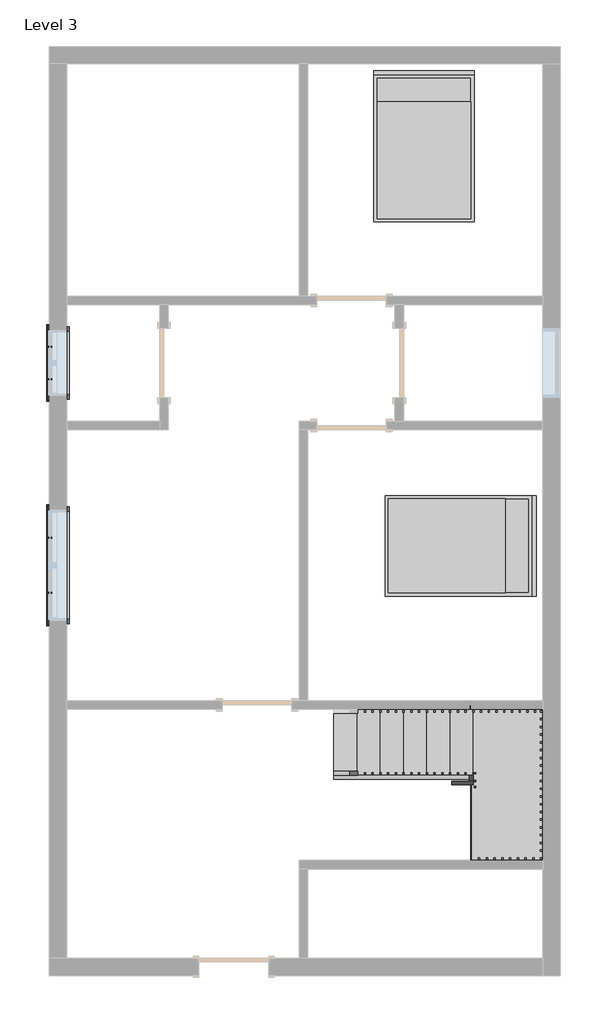
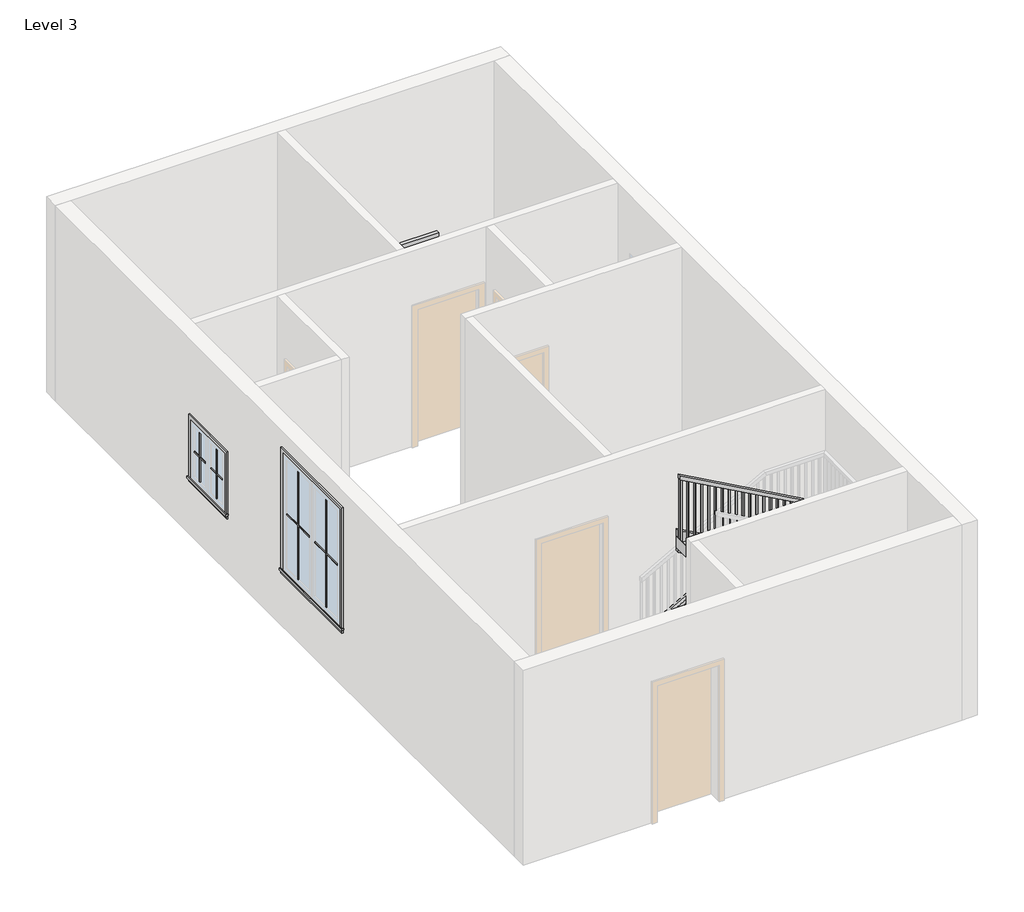
# One storey, part 2 of 2: 8 proxies, 6 members, 2 furniture elements, 1 railing, 1 stair flight.
"""IFC4 building model written with IfcOpenShell, lengths in millimetres."""

from ifc_helpers import new_model, si_unit, frame, origin, place, context, project, spatial, polyline, outline, extrude, faceted_brep, transform, mapped, element, save
from components import muntin_pattern_2x2_muntin_pattern_2x2_b3fe6957, muntin_pattern_2x2_muntin_pattern_2x2_3e0ecaf2, muntin_pattern_2x2_muntin_pattern_2x2_bff912c5, muntin_pattern_2x2_muntin_pattern_2x2_c2194282, trim_window_exterior_flat_with_sill_41619996, trim_window_exterior_flat_with_sill_e04b3088, trim_window_interior_flat_picture_frame_51c85655, trim_window_interior_flat_picture_frame_2a7685fe, bed_17739_bed_17739_15c61121, stair_flight_fe7d2e61

model = new_model("IFC4")

# Units and contexts
model_context = context("Model", 3, world=origin())
ifc_project = project(units=[si_unit("LENGTHUNIT", "METRE", prefix="MILLI")], contexts=[model_context])

# Site, building, storey
site = spatial("IfcSite", under=ifc_project)
building = spatial("IfcBuilding", under=site)
storey = spatial("IfcBuildingStorey", under=building, Name="Level 3", Elevation=3200.4)

# Proxies
placement = place(None, origin())
muntin_pattern_2x2_muntin_pattern_2x2_shape = muntin_pattern_2x2_muntin_pattern_2x2_b3fe6957(model_context)
element("IfcBuildingElementProxy", 1, Name="Muntin Pattern_2x2 : Muntin Pattern_2x2", ObjectType="Muntin Pattern_2x2 : Muntin Pattern_2x2", at=placement, inside=storey, context=model_context, shape_type="MappedRepresentation", body=[
    mapped(muntin_pattern_2x2_muntin_pattern_2x2_shape, transform((-4603.815747, 2266.9810985, 4184.65), x_axis=(0.0, 1.0, 0.0), y_axis=(-1.0, 0.0, 0.0), z_axis=(0.0, 0.0, 1.0))),
])
muntin_pattern_2x2_muntin_pattern_2x2_2_shape = muntin_pattern_2x2_muntin_pattern_2x2_3e0ecaf2(model_context)
element("IfcBuildingElementProxy", 2, Name="Muntin Pattern_2x2 : Muntin Pattern_2x2", ObjectType="Muntin Pattern_2x2 : Muntin Pattern_2x2", at=placement, inside=storey, context=model_context, shape_type="MappedRepresentation", body=[
    mapped(muntin_pattern_2x2_muntin_pattern_2x2_2_shape, transform((-4603.815747, 2695.6060985, 4184.65), x_axis=(0.0, -1.0, 0.0), y_axis=(1.0, 0.0, 0.0), z_axis=(0.0, 0.0, 1.0))),
])
muntin_pattern_2x2_muntin_pattern_2x2_3_shape = muntin_pattern_2x2_muntin_pattern_2x2_bff912c5(model_context)
element("IfcBuildingElementProxy", 3, Name="Muntin Pattern_2x2 : Muntin Pattern_2x2", ObjectType="Muntin Pattern_2x2 : Muntin Pattern_2x2", at=placement, inside=storey, context=model_context, shape_type="MappedRepresentation", body=[
    mapped(muntin_pattern_2x2_muntin_pattern_2x2_3_shape, transform((-4603.815747, -533.3689015, 4184.65), x_axis=(0.0, 1.0, 0.0), y_axis=(-1.0, 0.0, 0.0), z_axis=(0.0, 0.0, 1.0))),
])
muntin_pattern_2x2_muntin_pattern_2x2_4_shape = muntin_pattern_2x2_muntin_pattern_2x2_c2194282(model_context)
element("IfcBuildingElementProxy", 4, Name="Muntin Pattern_2x2 : Muntin Pattern_2x2", ObjectType="Muntin Pattern_2x2 : Muntin Pattern_2x2", at=placement, inside=storey, context=model_context, shape_type="MappedRepresentation", body=[
    mapped(muntin_pattern_2x2_muntin_pattern_2x2_4_shape, transform((-4603.815747, 187.3560985, 4184.65), x_axis=(0.0, -1.0, 0.0), y_axis=(1.0, 0.0, 0.0), z_axis=(0.0, 0.0, 1.0))),
])
trim_window_exterior_flat_with_sill_shape = trim_window_exterior_flat_with_sill_41619996(model_context)
element("IfcBuildingElementProxy", 5, Name="Trim-Window-Exterior-Flat : with Sill", ObjectType="Trim-Window-Exterior-Flat : with Sill", at=placement, inside=storey, context=model_context, shape_type="MappedRepresentation", body=[
    mapped(trim_window_exterior_flat_with_sill_shape, transform((-4613.340747, 2481.2935985, 5029.2), x_axis=(0.0, -1.0, 0.0), y_axis=(0.0, 0.0, 1.0), z_axis=(-1.0, 0.0, 0.0))),
])
trim_window_exterior_flat_with_sill_2_shape = trim_window_exterior_flat_with_sill_e04b3088(model_context)
element("IfcBuildingElementProxy", 6, Name="Trim-Window-Exterior-Flat : with Sill", ObjectType="Trim-Window-Exterior-Flat : with Sill", at=placement, inside=storey, context=model_context, shape_type="MappedRepresentation", body=[
    mapped(trim_window_exterior_flat_with_sill_2_shape, transform((-4613.340747, -173.0064015, 5943.6), x_axis=(0.0, -1.0, 0.0), y_axis=(0.0, 0.0, 1.0), z_axis=(-1.0, 0.0, 0.0))),
])
trim_window_interior_flat_picture_frame_shape = trim_window_interior_flat_picture_frame_51c85655(model_context)
element("IfcBuildingElementProxy", 7, Name="Trim-Window-Interior-Flat : Picture Frame", ObjectType="Trim-Window-Interior-Flat : Picture Frame", at=placement, inside=storey, context=model_context, shape_type="MappedRepresentation", body=[
    mapped(trim_window_interior_flat_picture_frame_shape, transform((-4384.740747, 2481.2935985, 5029.2), x_axis=(0.0, 1.0, 0.0), y_axis=(0.0, 0.0, 1.0), z_axis=(1.0, 0.0, 0.0))),
])
trim_window_interior_flat_picture_frame_2_shape = trim_window_interior_flat_picture_frame_2a7685fe(model_context)
element("IfcBuildingElementProxy", 8, Name="Trim-Window-Interior-Flat : Picture Frame", ObjectType="Trim-Window-Interior-Flat : Picture Frame", at=placement, inside=storey, context=model_context, shape_type="MappedRepresentation", body=[
    mapped(trim_window_interior_flat_picture_frame_2_shape, transform((-4384.740747, -173.0064015, 5943.6), x_axis=(0.0, 1.0, 0.0), y_axis=(0.0, 0.0, 1.0), z_axis=(1.0, 0.0, 0.0))),
])

# Furniture
bed_17739_bed_17739_shape = bed_17739_bed_17739_15c61121(model_context)
element("IfcFurniture", 9, ObjectType="Bed_17739 : Bed_17739", at=placement, inside=storey, context=model_context, shape_type="MappedRepresentation", body=[
    mapped(bed_17739_bed_17739_shape, transform((301.559253, 5300.6935985, 3200.4), x_axis=(1.0, 0.0, 0.0), y_axis=(0.0, 1.0, 0.0), z_axis=(0.0, 0.0, 1.0))),
])
element("IfcFurniture", 10, ObjectType="Bed_17739 : Bed_17739", at=placement, inside=storey, context=model_context, shape_type="MappedRepresentation", body=[
    mapped(bed_17739_bed_17739_shape, transform((758.759253, 80.9935985, 3200.4), x_axis=(0.0, -1.0, 0.0), y_axis=(1.0, 0.0, 0.0), z_axis=(0.0, 0.0, 1.0))),
])

# Members
element("IfcMember", 11, ObjectType="Stringer - 2\" Width", at=placement, inside=storey, context=model_context, shape_type="SweptSolid", body=[
    extrude(outline(polyline([(3407.9983948, -879.540747), (3200.4, -879.540747), (3200.4, -625.5962442), (4461.9333333, 1645.1637558), (4461.9333333, 1017.5421424), (3407.9983948, -879.540747)])), frame((0.0, -2065.3064015, 0.0), z_axis=(0.0, 1.0, 0.0), x_axis=(0.0, 0.0, 1.0)), (0.0, 0.0, 1.0), 50.8),
])
element("IfcMember", 12, ObjectType="Stringer - 2\" Width", at=placement, inside=storey, context=model_context, shape_type="SweptSolid", body=[
    extrude(outline(polyline([(1863.659253, -2014.5064015), (1914.459253, -2014.5064015), (1914.459253, -4046.5064015), (1863.659253, -4046.5064015), (1863.659253, -2014.5064015)])), frame((0.0, 0.0, 4157.1333333), z_axis=(0.0, 0.0, 1.0), x_axis=(1.0, 0.0, 0.0)), (0.0, 0.0, 1.0), 304.8),
])
element("IfcMember", 13, ObjectType="Stringer - 2\" Width", at=placement, inside=storey, context=model_context, shape_type="SweptSolid", body=[
    extrude(outline(polyline([(4157.1333333, 1734.4163636), (5609.3317281, -879.540747), (5260.653054, -879.540747), (4157.1333333, 1106.7947502), (4157.1333333, 1734.4163636)])), frame((0.0, -4097.3064015, 0.0), z_axis=(0.0, 1.0, 0.0), x_axis=(0.0, 0.0, 1.0)), (0.0, 0.0, 1.0), 50.8),
])
element("IfcMember", 14, ObjectType="Stringer - 2\" Width", at=placement, inside=storey, context=model_context, shape_type="SweptSolid", body=[
    extrude(outline(polyline([(3407.9983948, -879.540747), (3200.4, -879.540747), (3200.4, -625.5962442), (4047.0974984, 898.459253), (4395.7761726, 898.459253), (3407.9983948, -879.540747)])), frame((0.0, -2979.7064015, 0.0), z_axis=(0.0, 1.0, 0.0), x_axis=(0.0, 0.0, 1.0)), (0.0, 0.0, 1.0), 50.8),
])
element("IfcMember", 15, ObjectType="Stringer - 2\" Width", at=placement, inside=storey, context=model_context, shape_type="SweptSolid", body=[
    extrude(outline(polyline([(898.459253, -2928.9064015), (949.259253, -2928.9064015), (949.259253, -3005.1064015), (898.459253, -3005.1064015), (898.459253, -2928.9064015)])), frame((0.0, 0.0, 4157.1333333), z_axis=(0.0, 0.0, 1.0), x_axis=(1.0, 0.0, 0.0)), (0.0, 0.0, 1.0), 304.8),
])
element("IfcMember", 16, ObjectType="Stringer - 2\" Width", at=placement, inside=storey, context=model_context, shape_type="SweptSolid", body=[
    extrude(outline(polyline([(4244.653054, 949.259253), (4593.3317281, 949.259253), (5609.3317281, -879.540747), (5260.653054, -879.540747), (4244.653054, 949.259253)])), frame((0.0, -3055.9064015, 0.0), z_axis=(0.0, 1.0, 0.0), x_axis=(0.0, 0.0, 1.0)), (0.0, 0.0, 1.0), 50.8),
])

# Railing
element("IfcRailing", 17, ObjectType="Handrail - Rectangular", at=placement, inside=storey, context=model_context, shape_type="SolidModel", body=[
    faceted_brep([(-879.540747, -2878.1064015, 4284.1333333), (-879.540747, -2878.1064015, 4226.020221), (-879.540747, -2928.9064015, 4226.020221), (-879.540747, -2928.9064015, 4284.1333333), (873.059253, -2878.1064015, 5257.8), (923.859253, -2878.1064015, 5227.9091099), (923.859253, -2928.9064015, 5227.9091099), (873.059253, -2928.9064015, 5257.8), (873.059253, -2878.1064015, 5300.1333333), (923.859253, -2878.1064015, 5249.3333333), (923.859253, -2928.9064015, 5249.3333333), (873.059253, -2928.9064015, 5300.1333333), (1000.059253, -2878.1064015, 5300.1333333), (1000.059253, -2878.1064015, 5249.3333333), (949.259253, -2928.9064015, 5249.3333333), (949.259253, -2928.9064015, 5300.1333333), (1000.059253, -3005.1064015, 5300.1333333), (1000.059253, -3005.1064015, 5249.3333333), (949.259253, -3005.1064015, 5249.3333333), (949.259253, -3005.1064015, 5300.1333333), (1000.059253, -3055.9064015, 5300.1333333), (949.259253, -3055.9064015, 5300.1333333), (949.259253, -3106.7064015, 5249.3333333), (1000.059253, -3106.7064015, 5249.3333333)], [[[0, 1, 2, 3]], [[1, 0, 4, 5]], [[2, 1, 5, 6]], [[3, 2, 6, 7]], [[0, 3, 7, 4]], [[5, 4, 8, 9]], [[6, 5, 9, 10]], [[7, 6, 10, 11]], [[4, 7, 11, 8]], [[9, 8, 12, 13]], [[10, 9, 13, 14]], [[11, 10, 14, 15]], [[8, 11, 15, 12]], [[13, 12, 16, 17]], [[14, 13, 17, 18]], [[15, 14, 18, 19]], [[12, 15, 19, 16]], [[20, 21, 22, 23]], [[17, 16, 20, 23]], [[18, 17, 23, 22]], [[19, 18, 22, 21]], [[16, 19, 21, 20]]]),
    faceted_brep([(1000.059253, -3055.9064015, 5300.1333333), (1000.059253, -3106.7064015, 5249.3333333), (949.259253, -3106.7064015, 5249.3333333), (949.259253, -3055.9064015, 5300.1333333), (1000.059253, -3055.9064015, 5441.2444444), (949.259253, -3055.9064015, 5411.3535543), (949.259253, -3106.7064015, 5411.3535543), (1000.059253, -3106.7064015, 5441.2444444)], [[[0, 1, 2, 3]], [[4, 5, 6, 7]], [[1, 0, 4, 7]], [[2, 1, 7, 6]], [[3, 2, 6, 5]], [[0, 3, 5, 4]]]),
    faceted_brep([(1000.059253, -3106.7064015, 5441.2444444), (949.259253, -3106.7064015, 5411.3535543), (949.259253, -3055.9064015, 5411.3535543), (1000.059253, -3055.9064015, 5441.2444444), (-879.540747, -3106.7064015, 6485.4666667), (-879.540747, -3055.9064015, 6485.4666667), (-879.540747, -3055.9064015, 6427.3535543), (-879.540747, -3106.7064015, 6427.3535543)], [[[0, 1, 2, 3]], [[4, 5, 6, 7]], [[1, 0, 4, 7]], [[2, 1, 7, 6]], [[3, 2, 6, 5]], [[0, 3, 5, 4]]]),
    extrude(outline(polyline([(6407.9507765, -844.615747), (6418.5341099, -863.665747), (5401.7333333, -863.665747), (5401.7333333, -844.615747), (6407.9507765, -844.615747)])), frame((0.0, -3090.8314015, 0.0), z_axis=(0.0, 1.0, 0.0), x_axis=(0.0, 0.0, 1.0)), (0.0, 0.0, 1.0), 19.05),
    extrude(outline(polyline([(6351.5063321, -743.015747), (6362.0896654, -762.065747), (5401.7333333, -762.065747), (5401.7333333, -743.015747), (6351.5063321, -743.015747)])), frame((0.0, -3090.8314015, 0.0), z_axis=(0.0, 1.0, 0.0), x_axis=(0.0, 0.0, 1.0)), (0.0, 0.0, 1.0), 19.05),
    extrude(outline(polyline([(6295.0618876, -641.415747), (6305.645221, -660.465747), (5401.7333333, -660.465747), (5401.7333333, -641.415747), (6295.0618876, -641.415747)])), frame((0.0, -3090.8314015, 0.0), z_axis=(0.0, 1.0, 0.0), x_axis=(0.0, 0.0, 1.0)), (0.0, 0.0, 1.0), 19.05),
    extrude(outline(polyline([(6238.6174432, -539.815747), (6249.2007765, -558.865747), (5232.4, -558.865747), (5232.4, -539.815747), (6238.6174432, -539.815747)])), frame((0.0, -3090.8314015, 0.0), z_axis=(0.0, 1.0, 0.0), x_axis=(0.0, 0.0, 1.0)), (0.0, 0.0, 1.0), 19.05),
    extrude(outline(polyline([(6182.1729988, -438.215747), (6192.7563321, -457.265747), (5232.4, -457.265747), (5232.4, -438.215747), (6182.1729988, -438.215747)])), frame((0.0, -3090.8314015, 0.0), z_axis=(0.0, 1.0, 0.0), x_axis=(0.0, 0.0, 1.0)), (0.0, 0.0, 1.0), 19.05),
    extrude(outline(polyline([(6125.7285543, -336.615747), (6136.3118876, -355.665747), (5232.4, -355.665747), (5232.4, -336.615747), (6125.7285543, -336.615747)])), frame((0.0, -3090.8314015, 0.0), z_axis=(0.0, 1.0, 0.0), x_axis=(0.0, 0.0, 1.0)), (0.0, 0.0, 1.0), 19.05),
    extrude(outline(polyline([(6069.2841099, -235.015747), (6079.8674432, -254.065747), (5063.0666667, -254.065747), (5063.0666667, -235.015747), (6069.2841099, -235.015747)])), frame((0.0, -3090.8314015, 0.0), z_axis=(0.0, 1.0, 0.0), x_axis=(0.0, 0.0, 1.0)), (0.0, 0.0, 1.0), 19.05),
    extrude(outline(polyline([(6012.8396654, -133.415747), (6023.4229988, -152.465747), (5063.0666667, -152.465747), (5063.0666667, -133.415747), (6012.8396654, -133.415747)])), frame((0.0, -3090.8314015, 0.0), z_axis=(0.0, 1.0, 0.0), x_axis=(0.0, 0.0, 1.0)), (0.0, 0.0, 1.0), 19.05),
    extrude(outline(polyline([(5956.395221, -31.815747), (5966.9785543, -50.865747), (5063.0666667, -50.865747), (5063.0666667, -31.815747), (5956.395221, -31.815747)])), frame((0.0, -3090.8314015, 0.0), z_axis=(0.0, 1.0, 0.0), x_axis=(0.0, 0.0, 1.0)), (0.0, 0.0, 1.0), 19.05),
    extrude(outline(polyline([(5899.9507765, 69.784253), (5910.5341099, 50.734253), (4893.7333333, 50.734253), (4893.7333333, 69.784253), (5899.9507765, 69.784253)])), frame((0.0, -3090.8314015, 0.0), z_axis=(0.0, 1.0, 0.0), x_axis=(0.0, 0.0, 1.0)), (0.0, 0.0, 1.0), 19.05),
    extrude(outline(polyline([(5843.5063321, 171.384253), (5854.0896654, 152.334253), (4893.7333333, 152.334253), (4893.7333333, 171.384253), (5843.5063321, 171.384253)])), frame((0.0, -3090.8314015, 0.0), z_axis=(0.0, 1.0, 0.0), x_axis=(0.0, 0.0, 1.0)), (0.0, 0.0, 1.0), 19.05),
    extrude(outline(polyline([(5787.0618876, 272.984253), (5797.645221, 253.934253), (4893.7333333, 253.934253), (4893.7333333, 272.984253), (5787.0618876, 272.984253)])), frame((0.0, -3090.8314015, 0.0), z_axis=(0.0, 1.0, 0.0), x_axis=(0.0, 0.0, 1.0)), (0.0, 0.0, 1.0), 19.05),
    extrude(outline(polyline([(5730.6174432, 374.584253), (5741.2007765, 355.534253), (4724.4, 355.534253), (4724.4, 374.584253), (5730.6174432, 374.584253)])), frame((0.0, -3090.8314015, 0.0), z_axis=(0.0, 1.0, 0.0), x_axis=(0.0, 0.0, 1.0)), (0.0, 0.0, 1.0), 19.05),
    extrude(outline(polyline([(5674.1729988, 476.184253), (5684.7563321, 457.134253), (4724.4, 457.134253), (4724.4, 476.184253), (5674.1729988, 476.184253)])), frame((0.0, -3090.8314015, 0.0), z_axis=(0.0, 1.0, 0.0), x_axis=(0.0, 0.0, 1.0)), (0.0, 0.0, 1.0), 19.05),
    extrude(outline(polyline([(5617.7285543, 577.784253), (5628.3118876, 558.734253), (4724.4, 558.734253), (4724.4, 577.784253), (5617.7285543, 577.784253)])), frame((0.0, -3090.8314015, 0.0), z_axis=(0.0, 1.0, 0.0), x_axis=(0.0, 0.0, 1.0)), (0.0, 0.0, 1.0), 19.05),
    extrude(outline(polyline([(5561.2841099, 679.384253), (5571.8674432, 660.334253), (4555.0666667, 660.334253), (4555.0666667, 679.384253), (5561.2841099, 679.384253)])), frame((0.0, -3090.8314015, 0.0), z_axis=(0.0, 1.0, 0.0), x_axis=(0.0, 0.0, 1.0)), (0.0, 0.0, 1.0), 19.05),
    extrude(outline(polyline([(5504.8396654, 780.984253), (5515.4229988, 761.934253), (4555.0666667, 761.934253), (4555.0666667, 780.984253), (5504.8396654, 780.984253)])), frame((0.0, -3090.8314015, 0.0), z_axis=(0.0, 1.0, 0.0), x_axis=(0.0, 0.0, 1.0)), (0.0, 0.0, 1.0), 19.05),
    extrude(outline(polyline([(5448.395221, 882.584253), (5458.9785543, 863.534253), (4555.0666667, 863.534253), (4555.0666667, 882.584253), (5448.395221, 882.584253)])), frame((0.0, -3090.8314015, 0.0), z_axis=(0.0, 1.0, 0.0), x_axis=(0.0, 0.0, 1.0)), (0.0, 0.0, 1.0), 19.05),
    extrude(outline(polyline([(965.134253, -2995.5814015), (984.184253, -2995.5814015), (984.184253, -3014.6314015), (965.134253, -3014.6314015), (965.134253, -2995.5814015)])), frame((0.0, 0.0, 4385.7333333), z_axis=(0.0, 0.0, 1.0), x_axis=(1.0, 0.0, 0.0)), (0.0, 0.0, 1.0), 863.6),
    extrude(outline(polyline([(939.734253, -2913.0314015), (939.734253, -2893.9814015), (958.784253, -2893.9814015), (958.784253, -2913.0314015), (939.734253, -2913.0314015)])), frame((0.0, 0.0, 4385.7333333), z_axis=(0.0, 0.0, 1.0), x_axis=(1.0, 0.0, 0.0)), (0.0, 0.0, 1.0), 863.6),
    extrude(outline(polyline([(5190.8674432, 857.184253), (5180.2841099, 838.134253), (4216.4, 838.134253), (4216.4, 857.184253), (5190.8674432, 857.184253)])), frame((0.0, -2913.0314015, 0.0), z_axis=(0.0, 1.0, 0.0), x_axis=(0.0, 0.0, 1.0)), (0.0, 0.0, 1.0), 19.05),
    extrude(outline(polyline([(5134.4229988, 755.584253), (5123.8396654, 736.534253), (4216.4, 736.534253), (4216.4, 755.584253), (5134.4229988, 755.584253)])), frame((0.0, -2913.0314015, 0.0), z_axis=(0.0, 1.0, 0.0), x_axis=(0.0, 0.0, 1.0)), (0.0, 0.0, 1.0), 19.05),
    extrude(outline(polyline([(5077.9785543, 653.984253), (5067.395221, 634.934253), (4216.4, 634.934253), (4216.4, 653.984253), (5077.9785543, 653.984253)])), frame((0.0, -2913.0314015, 0.0), z_axis=(0.0, 1.0, 0.0), x_axis=(0.0, 0.0, 1.0)), (0.0, 0.0, 1.0), 19.05),
    extrude(outline(polyline([(5021.5341099, 552.384253), (5010.9507765, 533.334253), (4047.0666667, 533.334253), (4047.0666667, 552.384253), (5021.5341099, 552.384253)])), frame((0.0, -2913.0314015, 0.0), z_axis=(0.0, 1.0, 0.0), x_axis=(0.0, 0.0, 1.0)), (0.0, 0.0, 1.0), 19.05),
    extrude(outline(polyline([(4965.0896654, 450.784253), (4954.5063321, 431.734253), (4047.0666667, 431.734253), (4047.0666667, 450.784253), (4965.0896654, 450.784253)])), frame((0.0, -2913.0314015, 0.0), z_axis=(0.0, 1.0, 0.0), x_axis=(0.0, 0.0, 1.0)), (0.0, 0.0, 1.0), 19.05),
    extrude(outline(polyline([(4908.645221, 349.184253), (4898.0618876, 330.134253), (4047.0666667, 330.134253), (4047.0666667, 349.184253), (4908.645221, 349.184253)])), frame((0.0, -2913.0314015, 0.0), z_axis=(0.0, 1.0, 0.0), x_axis=(0.0, 0.0, 1.0)), (0.0, 0.0, 1.0), 19.05),
    extrude(outline(polyline([(4852.2007765, 247.584253), (4841.6174432, 228.534253), (3877.7333333, 228.534253), (3877.7333333, 247.584253), (4852.2007765, 247.584253)])), frame((0.0, -2913.0314015, 0.0), z_axis=(0.0, 1.0, 0.0), x_axis=(0.0, 0.0, 1.0)), (0.0, 0.0, 1.0), 19.05),
    extrude(outline(polyline([(4795.7563321, 145.984253), (4785.1729988, 126.934253), (3877.7333333, 126.934253), (3877.7333333, 145.984253), (4795.7563321, 145.984253)])), frame((0.0, -2913.0314015, 0.0), z_axis=(0.0, 1.0, 0.0), x_axis=(0.0, 0.0, 1.0)), (0.0, 0.0, 1.0), 19.05),
    extrude(outline(polyline([(4739.3118876, 44.384253), (4728.7285543, 25.334253), (3877.7333333, 25.334253), (3877.7333333, 44.384253), (4739.3118876, 44.384253)])), frame((0.0, -2913.0314015, 0.0), z_axis=(0.0, 1.0, 0.0), x_axis=(0.0, 0.0, 1.0)), (0.0, 0.0, 1.0), 19.05),
    extrude(outline(polyline([(4682.8674432, -57.215747), (4672.2841099, -76.265747), (3708.4, -76.265747), (3708.4, -57.215747), (4682.8674432, -57.215747)])), frame((0.0, -2913.0314015, 0.0), z_axis=(0.0, 1.0, 0.0), x_axis=(0.0, 0.0, 1.0)), (0.0, 0.0, 1.0), 19.05),
    extrude(outline(polyline([(4626.4229988, -158.815747), (4615.8396654, -177.865747), (3708.4, -177.865747), (3708.4, -158.815747), (4626.4229988, -158.815747)])), frame((0.0, -2913.0314015, 0.0), z_axis=(0.0, 1.0, 0.0), x_axis=(0.0, 0.0, 1.0)), (0.0, 0.0, 1.0), 19.05),
    extrude(outline(polyline([(4569.9785543, -260.415747), (4559.395221, -279.465747), (3708.4, -279.465747), (3708.4, -260.415747), (4569.9785543, -260.415747)])), frame((0.0, -2913.0314015, 0.0), z_axis=(0.0, 1.0, 0.0), x_axis=(0.0, 0.0, 1.0)), (0.0, 0.0, 1.0), 19.05),
    extrude(outline(polyline([(4513.5341099, -362.015747), (4502.9507765, -381.065747), (3539.0666667, -381.065747), (3539.0666667, -362.015747), (4513.5341099, -362.015747)])), frame((0.0, -2913.0314015, 0.0), z_axis=(0.0, 1.0, 0.0), x_axis=(0.0, 0.0, 1.0)), (0.0, 0.0, 1.0), 19.05),
    extrude(outline(polyline([(4457.0896654, -463.615747), (4446.5063321, -482.665747), (3539.0666667, -482.665747), (3539.0666667, -463.615747), (4457.0896654, -463.615747)])), frame((0.0, -2913.0314015, 0.0), z_axis=(0.0, 1.0, 0.0), x_axis=(0.0, 0.0, 1.0)), (0.0, 0.0, 1.0), 19.05),
    extrude(outline(polyline([(4400.645221, -565.215747), (4390.0618876, -584.265747), (3539.0666667, -584.265747), (3539.0666667, -565.215747), (4400.645221, -565.215747)])), frame((0.0, -2913.0314015, 0.0), z_axis=(0.0, 1.0, 0.0), x_axis=(0.0, 0.0, 1.0)), (0.0, 0.0, 1.0), 19.05),
    extrude(outline(polyline([(4344.2007765, -666.815747), (4333.6174432, -685.865747), (3369.7333333, -685.865747), (3369.7333333, -666.815747), (4344.2007765, -666.815747)])), frame((0.0, -2913.0314015, 0.0), z_axis=(0.0, 1.0, 0.0), x_axis=(0.0, 0.0, 1.0)), (0.0, 0.0, 1.0), 19.05),
    extrude(outline(polyline([(4287.7563321, -768.415747), (4277.1729988, -787.465747), (3369.7333333, -787.465747), (3369.7333333, -768.415747), (4287.7563321, -768.415747)])), frame((0.0, -2913.0314015, 0.0), z_axis=(0.0, 1.0, 0.0), x_axis=(0.0, 0.0, 1.0)), (0.0, 0.0, 1.0), 19.05),
    extrude(outline(polyline([(965.134253, -3071.7814015), (984.184253, -3071.7814015), (984.184253, -3090.8314015), (965.134253, -3090.8314015), (965.134253, -3071.7814015)])), frame((0.0, 0.0, 4385.7333333), z_axis=(0.0, 0.0, 1.0), x_axis=(1.0, 0.0, 0.0)), (0.0, 0.0, 1.0), 863.6),
    extrude(outline(polyline([(965.134253, -2913.0314015), (965.134253, -2893.9814015), (984.184253, -2893.9814015), (984.184253, -2913.0314015), (965.134253, -2913.0314015)])), frame((0.0, 0.0, 4385.7333333), z_axis=(0.0, 0.0, 1.0), x_axis=(1.0, 0.0, 0.0)), (0.0, 0.0, 1.0), 863.6),
    extrude(outline(polyline([(6416.770221, -860.490747), (6427.3535543, -879.540747), (5401.7333333, -879.540747), (5401.7333333, -860.490747), (6416.770221, -860.490747)])), frame((0.0, -3090.8314015, 0.0), z_axis=(0.0, 1.0, 0.0), x_axis=(0.0, 0.0, 1.0)), (0.0, 0.0, 1.0), 19.05),
    extrude(outline(polyline([(4236.6035543, -860.490747), (4226.020221, -879.540747), (3369.7333333, -879.540747), (3369.7333333, -860.490747), (4236.6035543, -860.490747)])), frame((0.0, -2913.0314015, 0.0), z_axis=(0.0, 1.0, 0.0), x_axis=(0.0, 0.0, 1.0)), (0.0, 0.0, 1.0), 19.05),
])

# Stair flight
stair_flight_shape = stair_flight_fe7d2e61(model_context)
element("IfcStairFlight", 18, ObjectType="2\" Tread 1\" Nosing 1/4\" Riser", at=placement, inside=storey, context=model_context, shape_type="MappedRepresentation", body=[
    mapped(stair_flight_shape, transform((0.0, 0.0, 0.0), x_axis=(1.0, 0.0, 0.0), y_axis=(0.0, 1.0, 0.0), z_axis=(0.0, 0.0, 1.0))),
])

save(model, "model.ifc")

# Revit data of these elements
# Type "Muntin Pattern_2x2 : Muntin Pattern_2x2"
#   Width [instance default] = 4' - 0"
#   Thickness = 0' - 0 1/2"
#   Height [instance default] = 4' - 0"
#   Distance = 0' - 0 3/4"
#   Interior Material [instance default] = none
#   Exterior Material [instance default] = none
#   Default Elevation = 0
# Type "Trim-Window-Exterior-Flat : with Sill"
#   Trim Width = 0' - 2 1/4"
#   Trim Thickness_Picture Frame = 0' - 1 1/4"
#   Trim Thickness_with Sill = 0' - 0 3/4"
#   Sill Thickness = 0' - 1 1/4"
#   Opening Width [instance default] = 2' - 0"
#   Opening Height [instance default] = 3' - 0"
#   Default Elevation = 4' - 0"
#   Sill = yes
#   Picture Frame = no
#   Trim Material [instance default] = none
# Type "Trim-Window-Interior-Flat : Picture Frame"
#   Trim Thickness_Picture Frame = 0' - 1 1/4"
#   Trim Width = 0' - 2 1/4"
#   Trim Thickness_with Sill = 0' - 0 3/4"
#   Sill Thickness = 0' - 1 1/4"
#   Opening Width [instance default] = 2' - 0"
#   Opening Height [instance default] = 3' - 0"
#   Default Elevation = 4' - 0"
#   Sill = no
#   Picture Frame = yes
#   Trim Material [instance default] = none
# Type "Bed_17739 : Bed_17739"
#   Default Elevation = 0
# Type "Handrail - Rectangular"
#   Assembly Code = "C2010400"
#   built-in parameter 1008612 = 0.0416667 (stored number, unit not read)
#   built-in parameter 1008611 = 0.0416667 (stored number, unit not read)
#   built-in parameter 1008609 = 0.333333 (stored number, unit not read)
#   built-in parameter 1008604 = 0.166667 (stored number, unit not read)
#   built-in parameter 1008603 = 0.166667 (stored number, unit not read)
#   Railing Height = 3' - 0"
#   built-in parameter 1008630 = 2
#   built-in parameter 1008610 = 2
#   built-in parameter 1008618 = Baluster - Square : 3/4"
# Elements 1, 2 (IfcBuildingElementProxy, "Muntin Pattern_2x2 : Muntin Pattern_2x2")
#   Width = 0' - 11 5/8"
#   Height = 2' - 6 1/2"
#   Interior Material = Wood - Stained
#   Exterior Material = Clad - White
#   Phase Created = New Construction
#   Materials on its faces: "Clad - White", "Wood - Stained"
# Elements 3, 4 (IfcBuildingElementProxy, "Muntin Pattern_2x2 : Muntin Pattern_2x2")
#   Width = 1' - 11 1/8"
#   Height = 5' - 6 1/2"
#   Interior Material = Wood - Stained
#   Exterior Material = Clad - White
#   Phase Created = New Construction
#   Materials on its faces: "Clad - White", "Wood - Stained"
# Element 5 (IfcBuildingElementProxy, "Trim-Window-Exterior-Flat : with Sill")
#   Opening Width = 2' - 10"
#   Opening Height = 3' - 0"
#   Trim Material = Clad - White
#   Phase Created = New Construction
#   Materials on its faces: "Clad - White"
# Element 6 (IfcBuildingElementProxy, "Trim-Window-Exterior-Flat : with Sill")
#   Opening Width = 4' - 9"
#   Opening Height = 6' - 0"
#   Trim Material = Clad - White
#   Phase Created = New Construction
#   Materials on its faces: "Clad - White"
# Element 7 (IfcBuildingElementProxy, "Trim-Window-Interior-Flat : Picture Frame")
#   Opening Width = 2' - 10"
#   Opening Height = 3' - 0"
#   Trim Material = Wood - Stained
#   Phase Created = New Construction
#   Materials on its faces: "Wood - Stained"
# Element 8 (IfcBuildingElementProxy, "Trim-Window-Interior-Flat : Picture Frame")
#   Opening Width = 4' - 9"
#   Opening Height = 6' - 0"
#   Trim Material = Wood - Stained
#   Phase Created = New Construction
#   Materials on its faces: "Wood - Stained"
# Elements 9, 10 (IfcFurniture, "Bed_17739 : Bed_17739")
#   Phase Created = New Construction
#   Materials on its faces: "legs", "sheets", "bed frame", "Blanket"
# Elements 11, 12, 13, 14, 15, 16 (IfcMember, "Stringer - 2\" Width")
#   Phase Created = New Construction
# Element 17 (IfcRailing, "Handrail - Rectangular")
#   Phase Created = New Construction
# Element 18 (IfcStairFlight, "2\" Tread 1\" Nosing 1/4\" Riser")
#   Phase Created = New Construction
# Materials
#   "Clad - White": class "Wood", colour RGB 242 242 238, transparency 0, Cost = 0
#   "Wood - Stained": class "Wood", colour RGB 224 178 126, transparency 0, Cost = 0
#   "legs": colour RGB 90 73 37, transparency 0, Cost = 0
#   "sheets": colour RGB 200 195 176, transparency 0, Cost = 0
#   "bed frame": colour RGB 90 73 37, transparency 0, Cost = 0
#   "Blanket": class "System", colour RGB 59 0 1, transparency 0, Cost = 0
